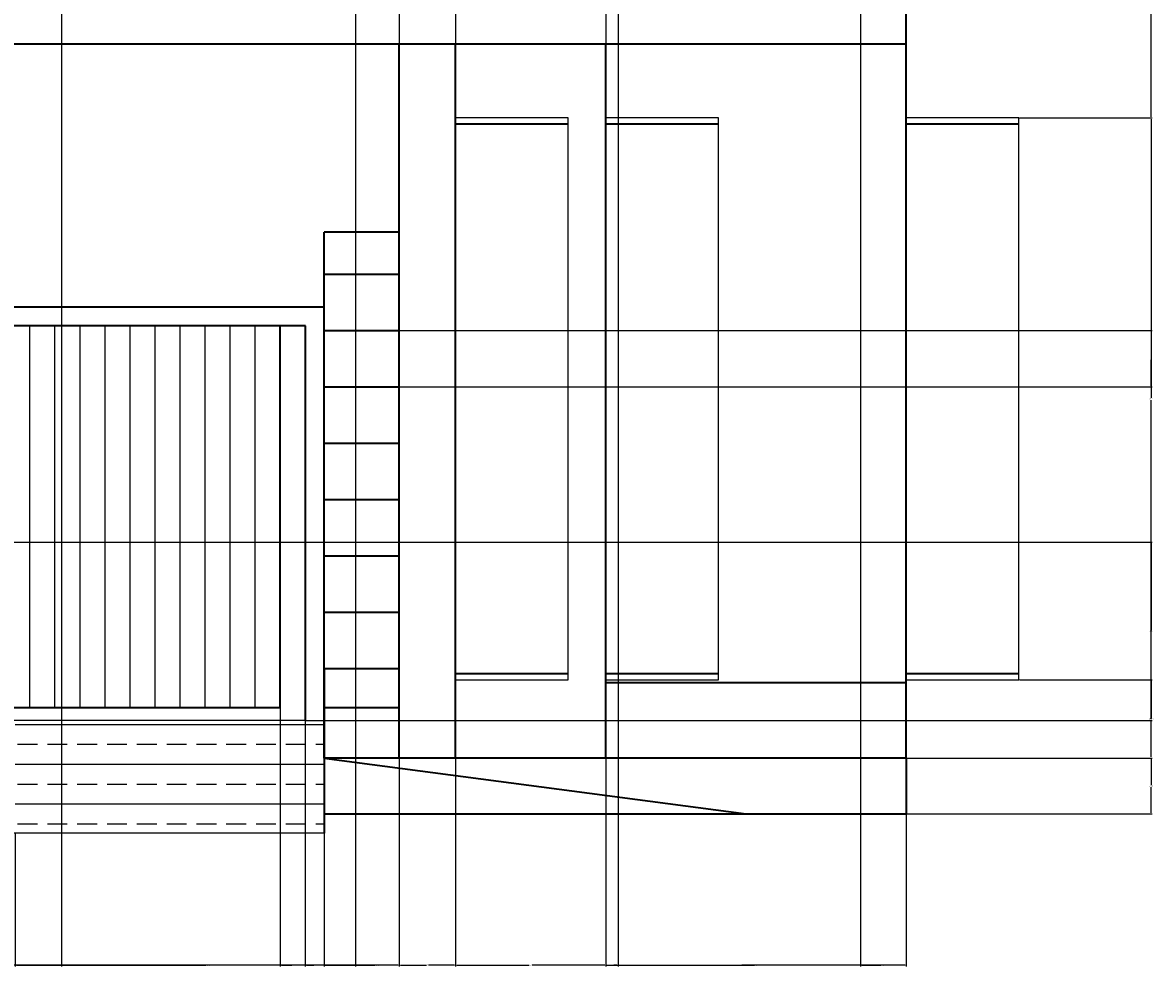
# Model space of a CAD drawing. Units: inches. Extents: x 2148 to 2587, y 1015 to 1466.
# Tile 3 of 7: x 2406 to 2587, y 1015 to 1166. Entities that reach past the tile are written whole.
import ezdxf

# ---------------------------------------------------------------- set-up
doc = ezdxf.new("R2010")
doc.units = ezdxf.units.IN
for name, color, linetype, lineweight in [('A-ANNO-DIMS', 2, 'Continuous', 18), ('A-DOOR', 3, 'Continuous', 25), ('A-ELEV', 7, 'Continuous', 35), ('A-FLOR-STRS', 2, 'Continuous', 25), ('A-GLAZ', 4, 'Continuous', 25)]:
    doc.layers.add(name, color=color, linetype=linetype, lineweight=lineweight)
doc.styles.get("Standard").update_dxf_attribs({"font": 'arial.ttf'})
doc.dimstyles.get("Standard").update_dxf_attribs({"dimtxt": 0.18, "dimasz": 0.18, "dimexe": 0.18, "dimexo": 0.0625, "dimgap": 0.09, "dimtad": 0, "dimtih": 1, "dimtoh": 1, "dimdec": 4, "dimzin": 0, "dimdsep": 46, "dimtxsty": 'Standard', "dimcen": 0.09, "dimadec": 0, "dimazin": 0, "dimtfac": 1, "dimtdec": 4, "dimtofl": 0, "dimtmove": 0, "dimatfit": 3, "dimfxl": 1, "dimtolj": 1, "dimtzin": 0, "dimarcsym": 0})

# ---------------------------------------------------------------- blocks, each defined once
blk = doc.blocks.new('WIN-SIDE')
for p, q in [((18, 89.73), (0, 89.73)), ((18, 0), (18, 89.73)), ((0, 0), (18, 0))]:
    blk.add_line(p, q)
blk = doc.blocks.new('*D12')
at = {"layer": 'A-ANNO-DIMS', "color": 0, "lineweight": -2, "transparency": 16777216}
for p, q in [((2316.03, 1162.68), (2316.03, 1015.46)), ((2466.03, 1048.68), (2466.03, 1015.46)), ((2316.21, 1015.64), (2390.75, 1015.64)), ((2465.85, 1015.64), (2391.31, 1015.64))]:
    blk.add_line(p, q, dxfattribs=at)
at = {"layer": 'A-ANNO-DIMS', "color": 0, "transparency": 16777216}
for points in [[(2316.21, 1015.67), (2316.21, 1015.61), (2316.03, 1015.64)], [(2465.85, 1015.67), (2465.85, 1015.61), (2466.03, 1015.64)]]:
    blk.add_solid(points, dxfattribs=at)
at = {"layer": 'Defpoints', "color": 0, "transparency": 16777216}
for p in [(2316.03, 1162.74), (2466.03, 1048.74), (2466.03, 1015.64)]:
    blk.add_point(p, dxfattribs=at)
at = {"layer": 'A-ANNO-DIMS', "color": 0, "transparency": 16777216, "insert": (2391.03, 1015.64), "char_height": 0.18, "attachment_point": 5}
blk.add_mtext('\\A1;150', dxfattribs=at)
blk = doc.blocks.new('*D13')
at = {"layer": 'A-ANNO-DIMS', "color": 0, "lineweight": -2, "transparency": 16777216}
for p, q in [((2466.03, 1048.68), (2466.03, 1015.46)), ((2475.03, 1048.68), (2475.03, 1015.46)), ((2466.21, 1015.64), (2470.39, 1015.64)), ((2474.85, 1015.64), (2470.68, 1015.64))]:
    blk.add_line(p, q, dxfattribs=at)
at = {"layer": 'A-ANNO-DIMS', "color": 0, "transparency": 16777216}
for points in [[(2466.21, 1015.67), (2466.21, 1015.61), (2466.03, 1015.64)], [(2474.85, 1015.67), (2474.85, 1015.61), (2475.03, 1015.64)]]:
    blk.add_solid(points, dxfattribs=at)
at = {"layer": 'Defpoints', "color": 0, "transparency": 16777216}
for p in [(2466.03, 1048.74), (2475.03, 1048.74), (2475.03, 1015.64)]:
    blk.add_point(p, dxfattribs=at)
at = {"layer": 'A-ANNO-DIMS', "color": 0, "transparency": 16777216, "insert": (2470.53, 1015.64), "char_height": 0.18, "attachment_point": 5}
blk.add_mtext('\\A1;9', dxfattribs=at)
blk = doc.blocks.new('*D14')
at = {"layer": 'A-ANNO-DIMS', "color": 0, "lineweight": -2, "transparency": 16777216}
for p, q in [((2475.03, 1048.68), (2475.03, 1015.46)), ((2499.03, 1048.68), (2499.03, 1015.46)), ((2475.21, 1015.64), (2486.81, 1015.64)), ((2498.85, 1015.64), (2487.25, 1015.64))]:
    blk.add_line(p, q, dxfattribs=at)
at = {"layer": 'A-ANNO-DIMS', "color": 0, "transparency": 16777216}
for points in [[(2475.21, 1015.67), (2475.21, 1015.61), (2475.03, 1015.64)], [(2498.85, 1015.67), (2498.85, 1015.61), (2499.03, 1015.64)]]:
    blk.add_solid(points, dxfattribs=at)
at = {"layer": 'Defpoints', "color": 0, "transparency": 16777216}
for p in [(2475.03, 1048.74), (2499.03, 1048.74), (2499.03, 1015.64)]:
    blk.add_point(p, dxfattribs=at)
at = {"layer": 'A-ANNO-DIMS', "color": 0, "transparency": 16777216, "insert": (2487.03, 1015.64), "char_height": 0.18, "attachment_point": 5}
blk.add_mtext('\\A1;24', dxfattribs=at)
blk = doc.blocks.new('*D15')
at = {"layer": 'A-ANNO-DIMS', "color": 0, "lineweight": -2, "transparency": 16777216}
for p, q in [((2499.03, 1048.68), (2499.03, 1015.46)), ((2547.03, 1039.75), (2547.03, 1015.46)), ((2499.21, 1015.64), (2522.81, 1015.64)), ((2546.85, 1015.64), (2523.26, 1015.64))]:
    blk.add_line(p, q, dxfattribs=at)
at = {"layer": 'A-ANNO-DIMS', "color": 0, "transparency": 16777216}
for points in [[(2499.21, 1015.67), (2499.21, 1015.61), (2499.03, 1015.64)], [(2546.85, 1015.67), (2546.85, 1015.61), (2547.03, 1015.64)]]:
    blk.add_solid(points, dxfattribs=at)
at = {"layer": 'Defpoints', "color": 0, "transparency": 16777216}
for p in [(2499.03, 1048.74), (2547.03, 1039.82), (2547.03, 1015.64)]:
    blk.add_point(p, dxfattribs=at)
at = {"layer": 'A-ANNO-DIMS', "color": 0, "transparency": 16777216, "insert": (2523.03, 1015.64), "char_height": 0.18, "attachment_point": 5}
blk.add_mtext('\\A1;48', dxfattribs=at)
blk = doc.blocks.new('*D27')
at = {"layer": 'A-ANNO-DIMS', "color": 0, "lineweight": -2, "transparency": 16777216}
for p, q in [((2547.1, 1048.74), (2586.31, 1048.74)), ((2586.13, 1048.56), (2586.13, 1044.46)), ((2586.13, 1040), (2586.13, 1044.1)), ((2547.1, 1039.82), (2586.31, 1039.82))]:
    blk.add_line(p, q, dxfattribs=at)
at = {"layer": 'A-ANNO-DIMS', "color": 0, "transparency": 16777216}
for points in [[(2586.1, 1048.56), (2586.16, 1048.56), (2586.13, 1048.74)], [(2586.1, 1040), (2586.16, 1040), (2586.13, 1039.82)]]:
    blk.add_solid(points, dxfattribs=at)
at = {"layer": 'Defpoints', "color": 0, "transparency": 16777216}
for p in [(2547.03, 1048.74), (2586.13, 1048.74), (2547.03, 1039.82)]:
    blk.add_point(p, dxfattribs=at)
at = {"layer": 'A-ANNO-DIMS', "color": 0, "transparency": 16777216, "insert": (2586.13, 1044.28), "char_height": 0.18, "attachment_point": 5}
blk.add_mtext('\\A1;8.925', dxfattribs=at)
blk = doc.blocks.new('*D28')
at = {"layer": 'A-ANNO-DIMS', "color": 0, "lineweight": -2, "transparency": 16777216}
for p, q in [((2565.1, 1061.24), (2586.31, 1061.24)), ((2586.13, 1061.06), (2586.13, 1055.17)), ((2586.13, 1048.92), (2586.13, 1054.81)), ((2547.1, 1048.74), (2586.31, 1048.74))]:
    blk.add_line(p, q, dxfattribs=at)
at = {"layer": 'A-ANNO-DIMS', "color": 0, "transparency": 16777216}
for points in [[(2586.1, 1061.06), (2586.16, 1061.06), (2586.13, 1061.24)], [(2586.1, 1048.92), (2586.16, 1048.92), (2586.13, 1048.74)]]:
    blk.add_solid(points, dxfattribs=at)
at = {"layer": 'Defpoints', "color": 0, "transparency": 16777216}
for p in [(2565.03, 1061.24), (2586.13, 1061.24), (2547.03, 1048.74)]:
    blk.add_point(p, dxfattribs=at)
at = {"layer": 'A-ANNO-DIMS', "color": 0, "transparency": 16777216, "insert": (2586.13, 1054.99), "char_height": 0.18, "attachment_point": 5}
blk.add_mtext('\\A1;12.498', dxfattribs=at)
blk = doc.blocks.new('*D29')
at = {"layer": 'A-ANNO-DIMS', "color": 0, "lineweight": -2, "transparency": 16777216}
for p, q in [((2565.1, 1150.97), (2586.31, 1150.97)), ((2586.13, 1150.79), (2586.13, 1106.29)), ((2586.13, 1061.42), (2586.13, 1105.92)), ((2565.1, 1061.24), (2586.31, 1061.24))]:
    blk.add_line(p, q, dxfattribs=at)
at = {"layer": 'A-ANNO-DIMS', "color": 0, "transparency": 16777216}
for points in [[(2586.1, 1150.79), (2586.16, 1150.79), (2586.13, 1150.97)], [(2586.1, 1061.42), (2586.16, 1061.42), (2586.13, 1061.24)]]:
    blk.add_solid(points, dxfattribs=at)
at = {"layer": 'Defpoints', "color": 0, "transparency": 16777216}
for p in [(2565.03, 1150.97), (2586.13, 1150.97), (2565.03, 1061.24)]:
    blk.add_point(p, dxfattribs=at)
at = {"layer": 'A-ANNO-DIMS', "color": 0, "transparency": 16777216, "insert": (2586.13, 1106.11), "char_height": 0.18, "attachment_point": 5}
blk.add_mtext('\\A1;89.73', dxfattribs=at)
blk = doc.blocks.new('*D30')
at = {"layer": 'A-ANNO-DIMS', "color": 0, "lineweight": -2, "transparency": 16777216}
for p, q in [((2565.1, 1215.74), (2586.31, 1215.74)), ((2586.13, 1215.56), (2586.13, 1183.54)), ((2586.13, 1151.15), (2586.13, 1183.18)), ((2565.1, 1150.97), (2586.31, 1150.97))]:
    blk.add_line(p, q, dxfattribs=at)
at = {"layer": 'A-ANNO-DIMS', "color": 0, "transparency": 16777216}
for points in [[(2586.1, 1215.56), (2586.16, 1215.56), (2586.13, 1215.74)], [(2586.1, 1151.15), (2586.16, 1151.15), (2586.13, 1150.97)]]:
    blk.add_solid(points, dxfattribs=at)
at = {"layer": 'Defpoints', "color": 0, "transparency": 16777216}
for p in [(2565.03, 1215.74), (2586.13, 1215.74), (2565.03, 1150.97)]:
    blk.add_point(p, dxfattribs=at)
at = {"layer": 'A-ANNO-DIMS', "color": 0, "transparency": 16777216, "insert": (2586.13, 1183.36), "char_height": 0.18, "attachment_point": 5}
blk.add_mtext('\\A1;64.77', dxfattribs=at)
blk = doc.blocks.new('*D50')
at = {"layer": 'A-ANNO-DIMS', "color": 0, "lineweight": -2, "transparency": 16777216}
for p, q in [((2365.07, 1174.68), (2365.07, 1015.46)), ((2412.06, 1174.68), (2412.06, 1015.46)), ((2365.25, 1015.64), (2388.16, 1015.64)), ((2411.88, 1015.64), (2388.96, 1015.64))]:
    blk.add_line(p, q, dxfattribs=at)
at = {"layer": 'A-ANNO-DIMS', "color": 0, "transparency": 16777216}
for points in [[(2365.25, 1015.67), (2365.25, 1015.61), (2365.07, 1015.64)], [(2411.88, 1015.67), (2411.88, 1015.61), (2412.06, 1015.64)]]:
    blk.add_solid(points, dxfattribs=at)
at = {"layer": 'Defpoints', "color": 0, "transparency": 16777216}
for p in [(2365.07, 1174.74), (2412.06, 1174.74), (2412.06, 1015.64)]:
    blk.add_point(p, dxfattribs=at)
at = {"layer": 'A-ANNO-DIMS', "color": 0, "transparency": 16777216, "insert": (2388.56, 1015.64), "char_height": 0.18, "attachment_point": 5}
blk.add_mtext('\\A1;46.99', dxfattribs=at)
blk = doc.blocks.new('*D51')
at = {"layer": 'A-ANNO-DIMS', "color": 0, "lineweight": -2, "transparency": 16777216}
for p, q in [((2412.06, 1174.68), (2412.06, 1015.46)), ((2459.04, 1174.68), (2459.04, 1015.46)), ((2412.24, 1015.64), (2435.15, 1015.64)), ((2458.86, 1015.64), (2435.95, 1015.64))]:
    blk.add_line(p, q, dxfattribs=at)
at = {"layer": 'A-ANNO-DIMS', "color": 0, "transparency": 16777216}
for points in [[(2412.24, 1015.67), (2412.24, 1015.61), (2412.06, 1015.64)], [(2458.86, 1015.67), (2458.86, 1015.61), (2459.04, 1015.64)]]:
    blk.add_solid(points, dxfattribs=at)
at = {"layer": 'Defpoints', "color": 0, "transparency": 16777216}
for p in [(2412.06, 1174.74), (2459.04, 1174.74), (2459.04, 1015.64)]:
    blk.add_point(p, dxfattribs=at)
at = {"layer": 'A-ANNO-DIMS', "color": 0, "transparency": 16777216, "insert": (2435.55, 1015.64), "char_height": 0.18, "attachment_point": 5}
blk.add_mtext('\\A1;46.99', dxfattribs=at)
blk = doc.blocks.new('*D52')
at = {"layer": 'A-ANNO-DIMS', "color": 0, "lineweight": -2, "transparency": 16777216}
for p, q in [((2466.03, 1329.68), (2466.03, 1015.46)), ((2459.04, 1174.68), (2459.04, 1015.46)), ((2459.22, 1015.64), (2462.14, 1015.64)), ((2465.85, 1015.64), (2462.93, 1015.64))]:
    blk.add_line(p, q, dxfattribs=at)
at = {"layer": 'A-ANNO-DIMS', "color": 0, "transparency": 16777216}
for points in [[(2459.22, 1015.67), (2459.22, 1015.61), (2459.04, 1015.64)], [(2465.85, 1015.67), (2465.85, 1015.61), (2466.03, 1015.64)]]:
    blk.add_solid(points, dxfattribs=at)
at = {"layer": 'Defpoints', "color": 0, "transparency": 16777216}
for p in [(2466.03, 1329.74), (2459.04, 1174.74), (2466.03, 1015.64)]:
    blk.add_point(p, dxfattribs=at)
at = {"layer": 'A-ANNO-DIMS', "color": 0, "transparency": 16777216, "insert": (2462.54, 1015.64), "char_height": 0.18, "attachment_point": 5}
blk.add_mtext('\\A1;6.993', dxfattribs=at)
blk = doc.blocks.new('*D53')
at = {"layer": 'A-ANNO-DIMS', "color": 0, "lineweight": -2, "transparency": 16777216}
for p, q in [((2475.03, 1351.68), (2475.03, 1015.46)), ((2466.03, 1329.68), (2466.03, 1015.46)), ((2466.21, 1015.64), (2470.39, 1015.64)), ((2474.85, 1015.64), (2470.68, 1015.64))]:
    blk.add_line(p, q, dxfattribs=at)
at = {"layer": 'A-ANNO-DIMS', "color": 0, "transparency": 16777216}
for points in [[(2466.21, 1015.67), (2466.21, 1015.61), (2466.03, 1015.64)], [(2474.85, 1015.67), (2474.85, 1015.61), (2475.03, 1015.64)]]:
    blk.add_solid(points, dxfattribs=at)
at = {"layer": 'Defpoints', "color": 0, "transparency": 16777216}
for p in [(2475.03, 1351.74), (2466.03, 1329.74), (2475.03, 1015.64)]:
    blk.add_point(p, dxfattribs=at)
at = {"layer": 'A-ANNO-DIMS', "color": 0, "transparency": 16777216, "insert": (2470.53, 1015.64), "char_height": 0.18, "attachment_point": 5}
blk.add_mtext('\\A1;9', dxfattribs=at)
blk = doc.blocks.new('*D54')
at = {"layer": 'A-ANNO-DIMS', "color": 0, "lineweight": -2, "transparency": 16777216}
for p, q in [((2475.03, 1351.68), (2475.03, 1015.46)), ((2499.03, 1329.68), (2499.03, 1015.46)), ((2475.21, 1015.64), (2486.81, 1015.64)), ((2498.85, 1015.64), (2487.25, 1015.64))]:
    blk.add_line(p, q, dxfattribs=at)
at = {"layer": 'A-ANNO-DIMS', "color": 0, "transparency": 16777216}
for points in [[(2475.21, 1015.67), (2475.21, 1015.61), (2475.03, 1015.64)], [(2498.85, 1015.67), (2498.85, 1015.61), (2499.03, 1015.64)]]:
    blk.add_solid(points, dxfattribs=at)
at = {"layer": 'Defpoints', "color": 0, "transparency": 16777216}
for p in [(2475.03, 1351.74), (2499.03, 1329.74), (2499.03, 1015.64)]:
    blk.add_point(p, dxfattribs=at)
at = {"layer": 'A-ANNO-DIMS', "color": 0, "transparency": 16777216, "insert": (2487.03, 1015.64), "char_height": 0.18, "attachment_point": 5}
blk.add_mtext('\\A1;24', dxfattribs=at)
blk = doc.blocks.new('*D55')
at = {"layer": 'A-ANNO-DIMS', "color": 0, "lineweight": -2, "transparency": 16777216}
for p, q in [((2499.03, 1329.68), (2499.03, 1015.46)), ((2500.98, 1174.68), (2500.98, 1015.46)), ((2499.21, 1015.64), (2499.69, 1015.64)), ((2500.8, 1015.64), (2500.33, 1015.64))]:
    blk.add_line(p, q, dxfattribs=at)
at = {"layer": 'A-ANNO-DIMS', "color": 0, "transparency": 16777216}
for points in [[(2499.21, 1015.67), (2499.21, 1015.61), (2499.03, 1015.64)], [(2500.8, 1015.67), (2500.8, 1015.61), (2500.98, 1015.64)]]:
    blk.add_solid(points, dxfattribs=at)
at = {"layer": 'Defpoints', "color": 0, "transparency": 16777216}
for p in [(2499.03, 1329.74), (2500.98, 1174.74), (2500.98, 1015.64)]:
    blk.add_point(p, dxfattribs=at)
at = {"layer": 'A-ANNO-DIMS', "color": 0, "transparency": 16777216, "insert": (2500.01, 1015.64), "char_height": 0.18, "attachment_point": 5}
blk.add_mtext('\\A1;1.95', dxfattribs=at)
blk = doc.blocks.new('*D56')
at = {"layer": 'A-ANNO-DIMS', "color": 0, "lineweight": -2, "transparency": 16777216}
for p, q in [((2500.98, 1174.68), (2500.98, 1015.46)), ((2539.73, 1174.68), (2539.73, 1015.46)), ((2501.16, 1015.64), (2519.96, 1015.64)), ((2539.55, 1015.64), (2520.75, 1015.64))]:
    blk.add_line(p, q, dxfattribs=at)
at = {"layer": 'A-ANNO-DIMS', "color": 0, "transparency": 16777216}
for points in [[(2501.16, 1015.67), (2501.16, 1015.61), (2500.98, 1015.64)], [(2539.55, 1015.67), (2539.55, 1015.61), (2539.73, 1015.64)]]:
    blk.add_solid(points, dxfattribs=at)
at = {"layer": 'Defpoints', "color": 0, "transparency": 16777216}
for p in [(2500.98, 1174.74), (2539.73, 1174.74), (2539.73, 1015.64)]:
    blk.add_point(p, dxfattribs=at)
at = {"layer": 'A-ANNO-DIMS', "color": 0, "transparency": 16777216, "insert": (2520.36, 1015.64), "char_height": 0.18, "attachment_point": 5}
blk.add_mtext('\\A1;38.74', dxfattribs=at)
blk = doc.blocks.new('*D57')
at = {"layer": 'A-ANNO-DIMS', "color": 0, "lineweight": -2, "transparency": 16777216}
for p, q in [((2547.03, 1329.68), (2547.03, 1015.46)), ((2539.73, 1174.68), (2539.73, 1015.46)), ((2539.91, 1015.64), (2542.99, 1015.64)), ((2546.85, 1015.64), (2543.77, 1015.64))]:
    blk.add_line(p, q, dxfattribs=at)
at = {"layer": 'A-ANNO-DIMS', "color": 0, "transparency": 16777216}
for points in [[(2539.91, 1015.67), (2539.91, 1015.61), (2539.73, 1015.64)], [(2546.85, 1015.67), (2546.85, 1015.61), (2547.03, 1015.64)]]:
    blk.add_solid(points, dxfattribs=at)
at = {"layer": 'Defpoints', "color": 0, "transparency": 16777216}
for p in [(2547.03, 1329.74), (2539.73, 1174.74), (2547.03, 1015.64)]:
    blk.add_point(p, dxfattribs=at)
at = {"layer": 'A-ANNO-DIMS', "color": 0, "transparency": 16777216, "insert": (2543.38, 1015.64), "char_height": 0.18, "attachment_point": 5}
blk.add_mtext('\\A1;7.307', dxfattribs=at)
blk = doc.blocks.new('*D106')
at = {"layer": 'A-ANNO-DIMS', "color": 0, "lineweight": -2, "transparency": 16777216}
for p, q in [((2447.03, 1056.68), (2447.03, 1015.46)), ((2404.7, 1036.68), (2404.7, 1015.46)), ((2404.88, 1015.64), (2425.47, 1015.64)), ((2446.85, 1015.64), (2426.26, 1015.64))]:
    blk.add_line(p, q, dxfattribs=at)
at = {"layer": 'A-ANNO-DIMS', "color": 0, "transparency": 16777216}
for points in [[(2404.88, 1015.67), (2404.88, 1015.61), (2404.7, 1015.64)], [(2446.85, 1015.67), (2446.85, 1015.61), (2447.03, 1015.64)]]:
    blk.add_solid(points, dxfattribs=at)
at = {"layer": 'Defpoints', "color": 0, "transparency": 16777216}
for p in [(2447.03, 1056.74), (2404.7, 1036.74), (2447.03, 1015.64)]:
    blk.add_point(p, dxfattribs=at)
at = {"layer": 'A-ANNO-DIMS', "color": 0, "transparency": 16777216, "insert": (2425.86, 1015.64), "char_height": 0.18, "attachment_point": 5}
blk.add_mtext('\\A1;42.34', dxfattribs=at)
blk = doc.blocks.new('*D107')
at = {"layer": 'A-ANNO-DIMS', "color": 0, "lineweight": -2, "transparency": 16777216}
for p, q in [((2451.03, 1117.68), (2451.03, 1015.46)), ((2447.03, 1056.68), (2447.03, 1015.46)), ((2447.21, 1015.64), (2448.88, 1015.64)), ((2450.85, 1015.64), (2449.19, 1015.64))]:
    blk.add_line(p, q, dxfattribs=at)
at = {"layer": 'A-ANNO-DIMS', "color": 0, "transparency": 16777216}
for points in [[(2447.21, 1015.67), (2447.21, 1015.61), (2447.03, 1015.64)], [(2450.85, 1015.67), (2450.85, 1015.61), (2451.03, 1015.64)]]:
    blk.add_solid(points, dxfattribs=at)
at = {"layer": 'Defpoints', "color": 0, "transparency": 16777216}
for p in [(2451.03, 1117.74), (2447.03, 1056.74), (2451.03, 1015.64)]:
    blk.add_point(p, dxfattribs=at)
at = {"layer": 'A-ANNO-DIMS', "color": 0, "transparency": 16777216, "insert": (2449.03, 1015.64), "char_height": 0.18, "attachment_point": 5}
blk.add_mtext('\\A1;4', dxfattribs=at)
blk = doc.blocks.new('*D108')
at = {"layer": 'A-ANNO-DIMS', "color": 0, "lineweight": -2, "transparency": 16777216}
for p, q in [((2451.03, 1117.68), (2451.03, 1015.46)), ((2454.03, 1036.68), (2454.03, 1015.46)), ((2451.21, 1015.64), (2452.39, 1015.64)), ((2453.85, 1015.64), (2452.68, 1015.64))]:
    blk.add_line(p, q, dxfattribs=at)
at = {"layer": 'A-ANNO-DIMS', "color": 0, "transparency": 16777216}
for points in [[(2451.21, 1015.67), (2451.21, 1015.61), (2451.03, 1015.64)], [(2453.85, 1015.67), (2453.85, 1015.61), (2454.03, 1015.64)]]:
    blk.add_solid(points, dxfattribs=at)
at = {"layer": 'Defpoints', "color": 0, "transparency": 16777216}
for p in [(2451.03, 1117.74), (2454.03, 1036.74), (2454.03, 1015.64)]:
    blk.add_point(p, dxfattribs=at)
at = {"layer": 'A-ANNO-DIMS', "color": 0, "transparency": 16777216, "insert": (2452.53, 1015.64), "char_height": 0.18, "attachment_point": 5}
blk.add_mtext('\\A1;3', dxfattribs=at)
blk = doc.blocks.new('*D109')
at = {"layer": 'A-ANNO-DIMS', "color": 0, "lineweight": -2, "transparency": 16777216}
for p, q in [((2466.03, 1048.68), (2466.03, 1015.46)), ((2454.03, 1036.68), (2454.03, 1015.46)), ((2454.21, 1015.64), (2459.82, 1015.64)), ((2465.85, 1015.64), (2460.24, 1015.64))]:
    blk.add_line(p, q, dxfattribs=at)
at = {"layer": 'A-ANNO-DIMS', "color": 0, "transparency": 16777216}
for points in [[(2454.21, 1015.67), (2454.21, 1015.61), (2454.03, 1015.64)], [(2465.85, 1015.67), (2465.85, 1015.61), (2466.03, 1015.64)]]:
    blk.add_solid(points, dxfattribs=at)
at = {"layer": 'Defpoints', "color": 0, "transparency": 16777216}
for p in [(2466.03, 1048.74), (2454.03, 1036.74), (2466.03, 1015.64)]:
    blk.add_point(p, dxfattribs=at)
at = {"layer": 'A-ANNO-DIMS', "color": 0, "transparency": 16777216, "insert": (2460.03, 1015.64), "char_height": 0.18, "attachment_point": 5}
blk.add_mtext('\\A1;12', dxfattribs=at)
blk = doc.blocks.new('*D120')
at = {"layer": 'A-ANNO-DIMS', "color": 0, "lineweight": -2, "transparency": 16777216}
for p, q in [((2391.1, 1083.24), (2586.31, 1083.24)), ((2586.13, 1083.06), (2586.13, 1069.17)), ((2586.13, 1054.92), (2586.13, 1068.81)), ((2454.1, 1054.74), (2586.31, 1054.74))]:
    blk.add_line(p, q, dxfattribs=at)
at = {"layer": 'A-ANNO-DIMS', "color": 0, "transparency": 16777216}
for points in [[(2586.1, 1083.06), (2586.16, 1083.06), (2586.13, 1083.24)], [(2586.1, 1054.92), (2586.16, 1054.92), (2586.13, 1054.74)]]:
    blk.add_solid(points, dxfattribs=at)
at = {"layer": 'Defpoints', "color": 0, "transparency": 16777216}
for p in [(2391.03, 1083.24), (2586.13, 1083.24), (2454.03, 1054.74)]:
    blk.add_point(p, dxfattribs=at)
at = {"layer": 'A-ANNO-DIMS', "color": 0, "transparency": 16777216, "insert": (2586.13, 1068.99), "char_height": 0.18, "attachment_point": 5}
blk.add_mtext('\\A1;28.5', dxfattribs=at)
blk = doc.blocks.new('*D121')
at = {"layer": 'A-ANNO-DIMS', "color": 0, "lineweight": -2, "transparency": 16777216}
for p, q in [((2454.1, 1117.03), (2586.31, 1117.03)), ((2586.13, 1116.85), (2586.13, 1112.71)), ((2586.13, 1108.21), (2586.13, 1112.35)), ((2454.1, 1108.03), (2586.31, 1108.03))]:
    blk.add_line(p, q, dxfattribs=at)
at = {"layer": 'A-ANNO-DIMS', "color": 0, "transparency": 16777216}
for points in [[(2586.1, 1116.85), (2586.16, 1116.85), (2586.13, 1117.03)], [(2586.1, 1108.21), (2586.16, 1108.21), (2586.13, 1108.03)]]:
    blk.add_solid(points, dxfattribs=at)
at = {"layer": 'Defpoints', "color": 0, "transparency": 16777216}
for p in [(2454.03, 1117.03), (2586.13, 1117.03), (2454.03, 1108.03)]:
    blk.add_point(p, dxfattribs=at)
at = {"layer": 'A-ANNO-DIMS', "color": 0, "transparency": 16777216, "insert": (2586.13, 1112.53), "char_height": 0.18, "attachment_point": 5}
blk.add_mtext('\\A1;9', dxfattribs=at)

msp = doc.modelspace()

# ---------------------------------------------------------------- hatches: boundary and pattern name
at = {"layer": 'A-FLOR-STRS'}
h = msp.add_hatch(dxfattribs=at)
h.set_pattern_fill('BRASS', color=256)
h.paths.add_polyline_path([(2380.364, 1054.7427), (2331.0343, 1054.7427), (2328.0343, 1054.7427), (2328.0343, 1036.7427), (2380.364, 1036.7427)])
h.paths.add_polyline_path([(2454.0343, 1054.7427), (2451.0343, 1054.7427), (2404.6955, 1054.7427), (2404.6955, 1036.7427), (2454.0343, 1036.7427)])

# ---------------------------------------------------------------- linework, layer by layer
at = {"layer": 'A-DOOR'}
for p, q in [((2407.0343, 1056.7427), (2407.0343, 1117.7427)), ((2411.0343, 1056.7427), (2411.0343, 1117.7427)), ((2415.0343, 1056.7427), (2415.0343, 1117.7427)), ((2419.0343, 1056.7427), (2419.0343, 1117.7427)), ((2423.0343, 1056.7427), (2423.0343, 1117.7427)), ((2427.0343, 1056.7427), (2427.0343, 1117.7427)), ((2431.0343, 1056.7427), (2431.0343, 1117.7427)), ((2435.0343, 1056.7427), (2435.0343, 1117.7427)), ((2439.0343, 1056.7427), (2439.0343, 1117.7427)), ((2443.0343, 1056.7427), (2443.0343, 1117.7427))]:
    msp.add_line(p, q, dxfattribs=at)
at = {"layer": 'A-ELEV'}
for p, q in [((2547.0343, 1048.7427), (2547.0343, 1394.7427)), ((2547.0343, 1162.7427), (2187.0343, 1162.7427)), ((2466.0343, 1048.7427), (2466.0343, 1162.7427)), ((2475.0343, 1048.7427), (2475.0343, 1162.7427)), ((2499.0343, 1048.7427), (2499.0343, 1162.7427)), ((2493.0343, 1149.9716), (2475.0343, 1149.9716)), ((2517.0343, 1149.9716), (2499.0343, 1149.9716)), ((2565.0343, 1149.9716), (2547.0343, 1149.9716)), ((2466.0343, 1132.7427), (2454.0343, 1132.7427)), ((2454.0343, 1048.7427), (2454.0343, 1132.7427)), ((2454.0343, 1126.0305), (2466.0343, 1126.0305)), ((2454.0343, 1120.7427), (2328.0343, 1120.7427)), ((2451.0343, 1117.7427), (2331.0343, 1117.7427)), ((2447.0343, 1056.7427), (2447.0343, 1117.7427)), ((2451.0343, 1054.7427), (2451.0343, 1117.7427)), ((2454.0343, 1117.0305), (2466.0343, 1117.0305)), ((2454.0343, 1108.0305), (2466.0343, 1108.0305)), ((2454.0343, 1099.0305), (2466.0343, 1099.0305)), ((2454.0343, 1090.0305), (2466.0343, 1090.0305)), ((2454.0343, 1081.0305), (2466.0343, 1081.0305)), ((2454.0343, 1072.0305), (2466.0343, 1072.0305)), ((2454.0343, 1063.0305), (2466.0343, 1063.0305)), ((2454.0343, 1063.0305), (2454.0343, 1036.7427)), ((2475.0343, 1062.2408), (2493.0343, 1062.2408)), ((2499.0343, 1062.2408), (2517.0343, 1062.2408)), ((2547.0343, 1062.2408), (2565.0343, 1062.2408)), ((2547.0343, 1060.7427), (2499.0343, 1060.7427)), ((2447.0343, 1056.7427), (2391.0343, 1056.7427)), ((2466.0343, 1056.7427), (2454.0343, 1056.7427)), ((2547.0343, 1048.7427), (2454.0343, 1048.7427)), ((2454.0343, 1048.7427), (2521.4331, 1039.8173)), ((2547.0343, 1048.7427), (2547.0343, 1039.8173)), ((2454.0343, 1039.8173), (2547.0343, 1039.8173))]:
    msp.add_line(p, q, dxfattribs=at)
at = {"layer": 'A-FLOR-STRS'}
for p, q in [((2451.0343, 1054.7427), (2391.0343, 1054.7427)), ((2451.0343, 1054.7427), (2454.0343, 1054.7427)), ((2454.0343, 1036.7427), (2328.0343, 1036.7427))]:
    msp.add_line(p, q, dxfattribs=at)

# ---------------------------------------------------------------- block references
at = {"layer": 'A-GLAZ'}
for p in [(2475.034, 1061.2412), (2499.034, 1061.2412), (2547.034, 1061.2412)]:
    msp.add_blockref('WIN-SIDE', p, dxfattribs=at)

# ---------------------------------------------------------------- dimensions: what is measured, and where the dimension line sits
at = {"layer": 'A-ANNO-DIMS'}
for base, p1, p2, override, picture, middle in [((2475.0343, 1015.6427), (2466.0343, 1329.7427), (2475.0343, 1351.7427), {"dimdec": 0, "dimlfac": 1, "dimrnd": 0, "dimzin": 0, "dimdsep": 46, "dimlunit": 2}, '*D53', (2470.5343, 1015.6427)), ((2499.0343, 1015.6427), (2475.0343, 1351.7427), (2499.0343, 1329.7427), {"dimdec": 0, "dimlfac": 1, "dimrnd": 0, "dimzin": 0, "dimdsep": 46, "dimlunit": 2}, '*D54', (2487.0343, 1015.6427)), ((2466.0343, 1015.6427), (2459.0414, 1174.7427), (2466.0343, 1329.7427), {"dimdec": 3, "dimlfac": 1, "dimrnd": 0, "dimzin": 0, "dimdsep": 46, "dimlunit": 2}, '*D52', (2462.5378, 1015.6427)), ((2500.9841, 1015.6427), (2499.0343, 1329.7427), (2500.9841, 1174.7427), {"dimdec": 2, "dimlfac": 1, "dimrnd": 0, "dimzin": 0, "dimdsep": 46, "dimlunit": 2}, '*D55', (2500.0092, 1015.6427)), ((2547.03427, 1015.64266), (2539.72683, 1174.74266), (2547.03427, 1329.74266), {"dimdec": 3, "dimlfac": 1, "dimrnd": 0, "dimzin": 0, "dimdsep": 46, "dimlunit": 2}, '*D57', (2543.38055, 1015.64266)), ((2412.0554, 1015.6427), (2365.0695, 1174.7427), (2412.0554, 1174.7427), {"dimdec": 2, "dimlfac": 1, "dimrnd": 0, "dimzin": 0, "dimdsep": 46, "dimlunit": 2}, '*D50', (2388.5624, 1015.6427)), ((2459.0414, 1015.6427), (2412.0554, 1174.7427), (2459.0414, 1174.7427), {"dimdec": 2, "dimlfac": 1, "dimrnd": 0, "dimzin": 0, "dimdsep": 46, "dimlunit": 2}, '*D51', (2435.5484, 1015.6427)), ((2539.7268, 1015.6427), (2500.9841, 1174.7427), (2539.7268, 1174.7427), {"dimdec": 2, "dimlfac": 1, "dimrnd": 0, "dimzin": 0, "dimdsep": 46, "dimlunit": 2}, '*D56', (2520.3554, 1015.6427)), ((2466.0343, 1015.6427), (2316.0343, 1162.7427), (2466.0343, 1048.7427), {"dimdec": 0, "dimlfac": 1, "dimrnd": 0, "dimzin": 0, "dimdsep": 46, "dimlunit": 2}, '*D12', (2391.0343, 1015.6427)), ((2451.0343, 1015.6427), (2447.0343, 1056.7427), (2451.0343, 1117.7427), {"dimdec": 0, "dimlfac": 1, "dimrnd": 0, "dimzin": 0, "dimdsep": 46, "dimlunit": 2}, '*D107', (2449.0343, 1015.6427)), ((2454.0343, 1015.6427), (2451.0343, 1117.7427), (2454.0343, 1036.7427), {"dimdec": 0, "dimlfac": 1, "dimrnd": 0, "dimzin": 0, "dimdsep": 46, "dimlunit": 2}, '*D108', (2452.5343, 1015.6427)), ((2447.0343, 1015.6427), (2404.6955, 1036.7427), (2447.0343, 1056.7427), {"dimdec": 2, "dimlfac": 1, "dimrnd": 0, "dimzin": 0, "dimdsep": 46, "dimlunit": 2}, '*D106', (2425.8649, 1015.6427)), ((2466.0343, 1015.6427), (2454.0343, 1036.7427), (2466.0343, 1048.7427), {"dimdec": 0, "dimlfac": 1, "dimrnd": 0, "dimzin": 0, "dimdsep": 46, "dimlunit": 2}, '*D109', (2460.0343, 1015.6427)), ((2475.0343, 1015.6427), (2466.0343, 1048.7427), (2475.0343, 1048.7427), {"dimdec": 0, "dimlfac": 1, "dimrnd": 0, "dimzin": 0, "dimdsep": 46, "dimlunit": 2}, '*D13', (2470.5343, 1015.6427)), ((2499.0343, 1015.6427), (2475.0343, 1048.7427), (2499.0343, 1048.7427), {"dimdec": 0, "dimlfac": 1, "dimrnd": 0, "dimzin": 0, "dimdsep": 46, "dimlunit": 2}, '*D14', (2487.0343, 1015.6427)), ((2547.0343, 1015.6427), (2499.0343, 1048.7427), (2547.0343, 1039.8173), {"dimdec": 0, "dimlfac": 1, "dimrnd": 0, "dimzin": 0, "dimdsep": 46, "dimlunit": 2}, '*D15', (2523.0343, 1015.6427))]:
    dim = msp.add_linear_dim(base=base, p1=p1, p2=p2, dimstyle='Standard', override=override, dxfattribs=at)
    dim.commit()
    dim.dimension.update_dxf_attribs({"geometry": picture, "text_midpoint": middle})
for base, p1, p2, override, picture, middle in [((2586.1343, 1215.7427), (2565.0343, 1150.9716), (2565.0343, 1215.7427), {"dimdec": 2, "dimlfac": 1, "dimrnd": 0, "dimzin": 0, "dimdsep": 46, "dimlunit": 2}, '*D30', (2586.1343, 1183.3571)), ((2586.1343, 1150.9716), (2565.0343, 1061.2408), (2565.0343, 1150.9716), {"dimdec": 2, "dimlfac": 1, "dimrnd": 0, "dimzin": 0, "dimdsep": 46, "dimlunit": 2}, '*D29', (2586.1343, 1106.1062)), ((2586.1343, 1117.0305), (2454.0343, 1108.0305), (2454.0343, 1117.0305), {"dimdec": 0, "dimlfac": 1, "dimrnd": 0, "dimzin": 0, "dimdsep": 46, "dimlunit": 2}, '*D121', (2586.1343, 1112.5305)), ((2586.1343, 1083.2427), (2454.0343, 1054.7427), (2391.0343, 1083.2427), {"dimdec": 1, "dimlfac": 1, "dimrnd": 0, "dimzin": 0, "dimdsep": 46, "dimlunit": 2}, '*D120', (2586.1343, 1068.9927)), ((2586.1343, 1061.2408), (2547.0343, 1048.7427), (2565.0343, 1061.2408), {"dimdec": 3, "dimlfac": 1, "dimrnd": 0, "dimzin": 0, "dimdsep": 46, "dimlunit": 2}, '*D28', (2586.1343, 1054.9917)), ((2586.1343, 1048.7427), (2547.0343, 1039.8173), (2547.0343, 1048.7427), {"dimdec": 3, "dimlfac": 1, "dimrnd": 0, "dimzin": 0, "dimdsep": 46, "dimlunit": 2}, '*D27', (2586.1343, 1044.28))]:
    dim = msp.add_linear_dim(base=base, p1=p1, p2=p2, angle=90, dimstyle='Standard', override=override, dxfattribs=at)
    dim.commit()
    dim.dimension.update_dxf_attribs({"geometry": picture, "text_midpoint": middle})

doc.saveas('drawing.dxf')
